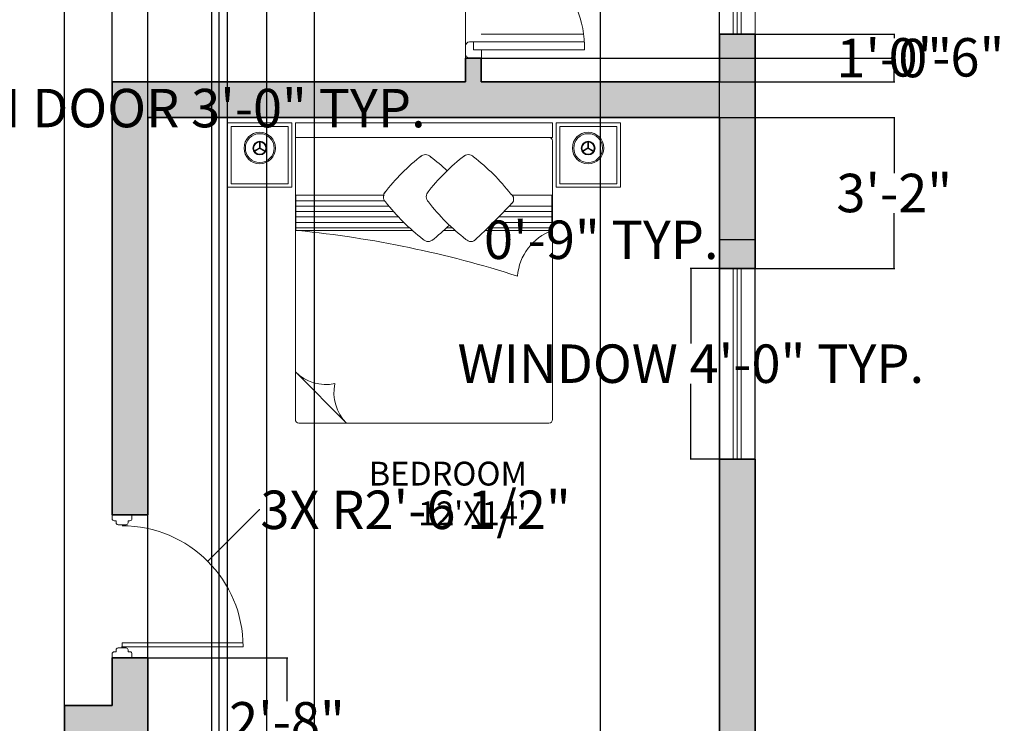
# Model space of a CAD drawing. Units: inches. Extents: x 2103 to 2702, y 2405 to 3142.
# Tile 4 of 7: x 2421 to 2669, y 2790 to 2968. Entities that reach past the tile are written whole.
import ezdxf

# ---------------------------------------------------------------- set-up
doc = ezdxf.new("R2010")
doc.units = ezdxf.units.IN
doc.linetypes.add('0', pattern=[0])
for name, color, linetype, lineweight in [('00 FURNITURE', 15, 'Continuous', 15), ('A-ANNO-DIMS', 2, 'Continuous', 18), ('A-AREA-IDEN', 7, 'Continuous', 18), ('A-WALL-PATT', 8, 'Continuous', 9), ('A_FUR 1', 5, 'Continuous', 5), ('doors', 4, 'Continuous', 18), ('WALL', 7, 'Continuous', 35), ('WINDOW', 160, '0', 5), ('windows', 4, 'Continuous', 18)]:
    doc.layers.add(name, color=color, linetype=linetype, lineweight=lineweight)
doc.layers.add('furniture', color=34, linetype='Continuous')
doc.styles.get("Standard").update_dxf_attribs({"font": 'arial.ttf'})
doc.dimstyles.get("Standard").update_dxf_attribs({"dimtxt": 9.68, "dimasz": 0.18, "dimexe": 0.18, "dimexo": 0.0625, "dimgap": 0.09, "dimtad": 0, "dimtih": 1, "dimtoh": 1, "dimdec": 1, "dimzin": 0, "dimdsep": 46, "dimlunit": 3, "dimtxsty": 'Standard', "dimcen": 0.09, "dimadec": 0, "dimazin": 0, "dimtfac": 1, "dimtdec": 1, "dimtofl": 0, "dimtmove": 0, "dimatfit": 3, "dimfxl": 1, "dimtolj": 1, "dimtzin": 0, "dimarcsym": 0})

# ---------------------------------------------------------------- blocks, each defined once
blk = doc.blocks.new('ESTSET')
at = {"layer": 'A_FUR 1'}
for p, q in [((-10.44, 4.1), (-10.44, 32.1)), ((-8.44, 4.1), (-8.44, 32.1)), ((-36.44, 6.1), (-36.44, 3.1)), ((-34.44, 6.1), (-36.44, 6.1)), ((-34.44, 4.1), (-34.44, 6.1)), ((-34.44, 4.1), (-34.44, 6.1)), ((-8.44, 4.1), (-8.44, 6.1)), ((-8.44, 6.1), (-6.44, 6.1)), ((-8.44, 4.1), (-8.44, 6.1)), ((-6.44, 6.1), (-6.44, 3.1)), ((-32.44, 4.1), (-34.44, 4.1)), ((-32.44, 4.1), (-34.44, 4.1)), ((-32.44, 3.1), (-32.44, 4.1)), ((-10.44, 3.1), (-10.44, 4.1)), ((-10.44, 4.1), (-8.44, 4.1)), ((-10.44, 4.1), (-8.44, 4.1)), ((-6.44, 2.1), (-36.44, 2.1)), ((-35.44, 2.1), (-33.44, 2.1)), ((-7.44, 2.1), (-9.44, 2.1))]:
    blk.add_line(p, q, dxfattribs=at)
for points in [[(-21.44, 2.1), (-18.67, 2.1), (-18.67, 5.1), (-20.06, 5.1)], [(-20.06, 5.1), (-20.06, -0.91)], [(-21.44, 2.1), (-21.44, -0.91), (-20.06, -0.91)]]:
    blk.add_lwpolyline(points, dxfattribs=at)
for centre, radius, start, end in [((-8.91, 6.46), 25.64, 88.9606, 185.2816), ((-35.44, 3.1), 1, 180, 270), ((-33.44, 3.1), 1, 270, 0), ((-9.44, 3.1), 1, 180, 270), ((-7.44, 3.1), 1, 270, 0)]:
    blk.add_arc(centre, radius, start, end, dxfattribs=at)
blk = doc.blocks.new('DDD')
at = {"layer": '00 FURNITURE'}
for p, q in [((-12579.77, -15859.53), (-12579.77, -15829.05)), ((-12578.77, -15859.53), (-12578.77, -15829.03)), ((-12612.02, -15857.03), (-12612.02, -15862.03)), ((-12611.02, -15857.03), (-12612.02, -15857.03)), ((-12610.52, -15858.03), (-12610.52, -15857.53)), ((-12577.52, -15858.03), (-12577.52, -15857.53)), ((-12577.02, -15857.03), (-12576.02, -15857.03)), ((-12576.02, -15857.03), (-12576.02, -15862.03)), ((-12578.77, -15859.53), (-12579.77, -15859.53)), ((-12612.02, -15862.03), (-12611.02, -15862.03)), ((-12610.52, -15861.53), (-12610.52, -15861.03)), ((-12577.52, -15861.53), (-12577.52, -15861.03)), ((-12576.02, -15862.03), (-12577.02, -15862.03))]:
    blk.add_line(p, q, dxfattribs=at)
for points in [[(-12610.52, -15861.03), (-12610.02, -15861.03, 0.414214), (-12609.52, -15860.53), (-12609.52, -15858.53, 0.414214), (-12610.02, -15858.03), (-12610.52, -15858.03)], [(-12577.52, -15861.03), (-12578.02, -15861.03, -0.414214), (-12578.52, -15860.53), (-12578.52, -15858.53, -0.414214), (-12578.02, -15858.03), (-12577.52, -15858.03)]]:
    blk.add_lwpolyline(points, format="xyb", dxfattribs=at)
for centre, radius, start, end in [((-12578.77, -15859.53), 30.5, 90, 180), ((-12611.02, -15857.53), 0.5, 0, 90), ((-12577.02, -15857.53), 0.5, 90, 180), ((-12611.02, -15861.53), 0.5, 270, 0), ((-12577.02, -15861.53), 0.5, 180, 270)]:
    blk.add_arc(centre, radius, start, end, dxfattribs=at)
blk = doc.blocks.new('window')
at = {"layer": 'furniture'}
for p, q in [((1745.13, 2764.08), (1745.13, 2716.08)), ((1754.13, 2716.08), (1754.13, 2764.08))]:
    blk.add_line(p, q, dxfattribs=at)
at = {"layer": 'WINDOW'}
for p, q in [((1748.63, 2764.08), (1748.63, 2716.08)), ((1749.63, 2764.08), (1749.63, 2716.08)), ((1750.63, 2764.08), (1750.63, 2716.08))]:
    blk.add_line(p, q, dxfattribs=at)
blk = doc.blocks.new('ventilator')
at = {"layer": 'windows'}
for p, q in [((1922.12, 2523.05), (1898.12, 2523.05)), ((1922.12, 2522.05), (1898.12, 2522.05)), ((1922.12, 2521.05), (1898.12, 2521.05))]:
    blk.add_line(p, q, dxfattribs=at)
blk.add_lwpolyline([(1898.12, 2526.55), (1898.12, 2517.55), (1922.12, 2517.55), (1922.12, 2526.55)], close=True, dxfattribs=at)
blk = doc.blocks.new('RGWTG')
at = {"layer": '00 FURNITURE'}
for p, q in [((578.23, 3473.51), (577.36, 3475.01)), ((578.23, 3473.58), (577.36, 3472.08)), ((578.36, 3473.58), (577.49, 3475.09)), ((578.36, 3473.51), (577.49, 3472)), ((578.29, 3473.62), (580.03, 3473.62)), ((578.29, 3473.47), (580.03, 3473.47)), ((521.93, 3464.58), (509.03, 3451.68)), ((509.03, 3422.63), (509.03, 3463.68)), ((509.93, 3464.58), (566.4, 3464.58)), ((557.53, 3463.84), (557.53, 3464.49)), ((557.53, 3464.49), (566.4, 3464.49)), ((558.2, 3464.49), (558.2, 3435.82)), ((559.57, 3464.49), (559.57, 3437.25)), ((560.94, 3464.49), (560.94, 3438.58)), ((562.3, 3464.49), (562.3, 3439.83)), ((563.67, 3464.49), (563.67, 3440.99)), ((565.04, 3464.49), (565.04, 3442.08)), ((566.4, 3464.58), (580.98, 3464.58)), ((566.4, 3464.49), (566.4, 3442.08)), ((566.4, 3464.49), (566.4, 3463.84)), ((580.98, 3464.58), (580.98, 3416.72)), ((558.2, 3426.48), (558.2, 3425.04)), ((509.03, 3400.68), (509.03, 3422.63)), ((558.2, 3416.13), (558.2, 3399.95)), ((580.98, 3416.72), (580.98, 3400.68)), ((559.57, 3414.75), (559.57, 3399.95)), ((560.94, 3413.39), (560.94, 3399.95)), ((562.3, 3412.04), (562.3, 3399.95)), ((563.67, 3410.72), (563.67, 3399.95)), ((580.08, 3399.78), (509.93, 3399.78)), ((557.53, 3399.95), (557.53, 3400.6)), ((566.4, 3399.95), (557.53, 3399.95)), ((566.4, 3400.6), (566.4, 3399.95)), ((578.23, 3390.78), (577.36, 3392.29)), ((578.36, 3390.86), (577.49, 3392.36)), ((578.23, 3390.86), (577.36, 3389.36)), ((578.36, 3390.78), (577.49, 3389.28)), ((578.29, 3390.9), (580.03, 3390.9)), ((578.29, 3390.74), (580.03, 3390.74))]:
    blk.add_line(p, q, dxfattribs=at)
for points in [[(568.43, 3465.48), (584.63, 3465.48), (584.63, 3481.68), (568.43, 3481.68)], [(569.33, 3466.38), (583.73, 3466.38), (583.73, 3480.78), (569.33, 3480.78)], [(580.98, 3399.78), (584.63, 3399.78), (584.63, 3464.58), (580.98, 3464.58)], [(568.43, 3398.88), (584.63, 3398.88), (584.63, 3382.68), (568.43, 3382.68)], [(569.33, 3397.98), (583.73, 3397.98), (583.73, 3383.58), (569.33, 3383.58)]]:
    blk.add_lwpolyline(points, close=True, dxfattribs=at)
for points in [[(566.52, 3464.49), (557.53, 3464.49), (557.53, 3435.08)], [(557.53, 3427.21), (557.53, 3424.3)], [(557.53, 3416.82), (557.53, 3399.95), (566.4, 3399.95), (566.4, 3409.94)]]:
    blk.add_lwpolyline(points, dxfattribs=at)
for centre, radius in [((578.29, 3473.54), 3.97), ((578.29, 3473.54), 3.63), ((578.29, 3473.54), 1.74), ((578.29, 3473.54), 1.56), ((578.29, 3390.82), 3.97), ((578.29, 3390.82), 3.63), ((578.29, 3390.82), 1.74), ((578.29, 3390.82), 1.56)]:
    blk.add_circle(centre, radius, dxfattribs=at)
for centre, radius, start, end in [((509.93, 3463.68), 0.9, 90, 180), ((529.65, 3456.88), 10.9, 135.0361, 191.9278), ((290.56, 3490.52), 268.3, 342.2214, 354.2925), ((516.73, 3443.97), 10.9, 78.0722, 134.9639), ((598.15, 3399.01), 54.32, 127.931, 142.069), ((566.05, 3440.57), 1.82, 45, 135), ((533.58, 3399.31), 54.32, 37.931, 52.069), ((556.59, 3431.11), 1.82, 135, 225), ((598.15, 3388.23), 54.32, 127.931, 142.069), ((566.05, 3429.78), 1.82, 45, 135), ((533.58, 3388.53), 54.32, 37.931, 52.069), ((574.84, 3431.77), 1.82, 315, 45), ((597.87, 3463.6), 54.32, 217.931, 224.141), ((533.28, 3463.88), 54.32, 316.32, 322.069), ((556.59, 3420.33), 1.82, 135, 225), ((574.84, 3420.99), 1.82, 315, 45), ((765.33, 3619.75), 290.45, 223.6069, 226.2326), ((533.28, 3453.1), 54.32, 307.931, 322.069), ((545.02, 3395.29), 13.35, 20.4224, 85.5825), ((565.44, 3411.05), 1.47, 225.9674, 326.8337), ((509.93, 3400.68), 0.9, 180, 270), ((580.08, 3400.68), 0.9, 270, 0)]:
    blk.add_arc(centre, radius, start, end, dxfattribs=at)
blk = doc.blocks.new('*D18')
at = {"layer": 'A-ANNO-DIMS', "color": 0, "lineweight": -2, "transparency": 16777216}
for p, q in [((2597.37, 2904.89), (2590.05, 2904.89)), ((2590.23, 2904.71), (2590.23, 2885.99)), ((2590.23, 2857.07), (2590.23, 2875.79)), ((2597.37, 2856.89), (2590.05, 2856.89))]:
    blk.add_line(p, q, dxfattribs=at)
at = {"layer": 'A-ANNO-DIMS', "color": 0, "transparency": 16777216}
for points in [[(2590.2, 2904.71), (2590.26, 2904.71), (2590.23, 2904.89)], [(2590.2, 2857.07), (2590.26, 2857.07), (2590.23, 2856.89)]]:
    blk.add_solid(points, dxfattribs=at)
at = {"layer": 'Defpoints', "color": 0, "transparency": 16777216}
for p in [(2597.43, 2904.89), (2590.23, 2856.89), (2597.43, 2856.89)]:
    blk.add_point(p, dxfattribs=at)
at = {"layer": 'A-ANNO-DIMS', "color": 0, "transparency": 16777216, "insert": (2590.23, 2880.89), "char_height": 9.68, "attachment_point": 5}
blk.add_mtext('\\A1;WINDOW 4\'-0" TYP.', dxfattribs=at)
blk = doc.blocks.new('*D19')
at = {"layer": 'A-ANNO-DIMS', "color": 0, "lineweight": -2, "transparency": 16777216}
for p, q in [((2597.43, 2904.95), (2597.43, 2912.27)), ((2606.43, 2904.95), (2606.43, 2912.27)), ((2597.43, 2912.09), (2597.25, 2912.09)), ((2606.25, 2912.09), (2597.61, 2912.09))]:
    blk.add_line(p, q, dxfattribs=at)
at = {"layer": 'A-ANNO-DIMS', "color": 0, "transparency": 16777216}
for points in [[(2597.61, 2912.12), (2597.61, 2912.06), (2597.43, 2912.09)], [(2606.25, 2912.12), (2606.25, 2912.06), (2606.43, 2912.09)]]:
    blk.add_solid(points, dxfattribs=at)
at = {"layer": 'Defpoints', "color": 0, "transparency": 16777216}
for p in [(2597.43, 2912.09), (2597.43, 2904.89), (2606.43, 2904.89)]:
    blk.add_point(p, dxfattribs=at)
at = {"layer": 'A-ANNO-DIMS', "color": 0, "transparency": 16777216, "insert": (2567.66, 2912.09), "char_height": 9.68, "attachment_point": 5}
blk.add_mtext('\\A1;0\'-9" TYP.', dxfattribs=at)
blk = doc.blocks.new('*D22')
at = {"layer": 'A-ANNO-DIMS', "color": 0, "lineweight": -2, "transparency": 16777216}
for p, q in [((2342.43, 2939.91), (2342.43, 2945.43)), ((2342.61, 2945.25), (2378.25, 2945.25)), ((2378.43, 2939.91), (2378.43, 2945.43)), ((2378.43, 2945.25), (2378.61, 2945.25))]:
    blk.add_line(p, q, dxfattribs=at)
at = {"layer": 'A-ANNO-DIMS', "color": 0, "transparency": 16777216}
for points in [[(2342.61, 2945.28), (2342.61, 2945.22), (2342.43, 2945.25)], [(2378.25, 2945.28), (2378.25, 2945.22), (2378.43, 2945.25)]]:
    blk.add_solid(points, dxfattribs=at)
at = {"layer": 'Defpoints', "color": 0, "transparency": 16777216}
for p in [(2378.43, 2945.25), (2342.43, 2939.85), (2378.43, 2939.85)]:
    blk.add_point(p, dxfattribs=at)
at = {"layer": 'A-ANNO-DIMS', "color": 0, "transparency": 16777216, "insert": (2453.03, 2945.25), "char_height": 9.68, "attachment_point": 5}
blk.add_mtext('\\A1;ROOM DOOR 3\'-0" TYP.', dxfattribs=at)
blk = doc.blocks.new('*D40')
at = {"layer": 'A-ANNO-DIMS', "color": 0, "lineweight": -2, "transparency": 16777216}
for p, q in [((2396.43, 2906.91), (2396.43, 3118.9)), ((2396.61, 3118.72), (2407.28, 3118.72)), ((2444.25, 3118.72), (2433.58, 3118.72)), ((2444.43, 2842.91), (2444.43, 3118.9))]:
    blk.add_line(p, q, dxfattribs=at)
at = {"layer": 'A-ANNO-DIMS', "color": 0, "transparency": 16777216}
for points in [[(2396.61, 3118.75), (2396.61, 3118.69), (2396.43, 3118.72)], [(2444.25, 3118.75), (2444.25, 3118.69), (2444.43, 3118.72)]]:
    blk.add_solid(points, dxfattribs=at)
at = {"layer": 'Defpoints', "color": 0, "transparency": 16777216}
for p in [(2444.43, 3118.72), (2396.43, 2906.85), (2444.43, 2842.85)]:
    blk.add_point(p, dxfattribs=at)
at = {"layer": 'A-ANNO-DIMS', "color": 0, "transparency": 16777216, "insert": (2420.43, 3118.72), "char_height": 9.68, "attachment_point": 5}
blk.add_mtext('\\A1;4\'-0"', dxfattribs=at)
blk = doc.blocks.new('*D44')
at = {"layer": 'A-ANNO-DIMS', "color": 0, "lineweight": -2, "transparency": 16777216}
for p, q in [((2471.43, 2560.91), (2471.43, 3118.9)), ((2471.61, 3118.72), (2483.25, 3118.72)), ((2483.43, 2560.91), (2483.43, 3118.9)), ((2483.43, 3118.72), (2483.61, 3118.72))]:
    blk.add_line(p, q, dxfattribs=at)
at = {"layer": 'A-ANNO-DIMS', "color": 0, "transparency": 16777216}
for points in [[(2471.61, 3118.75), (2471.61, 3118.69), (2471.43, 3118.72)], [(2483.25, 3118.75), (2483.25, 3118.69), (2483.43, 3118.72)]]:
    blk.add_solid(points, dxfattribs=at)
at = {"layer": 'Defpoints', "color": 0, "transparency": 16777216}
for p in [(2483.43, 3118.72), (2471.43, 2560.85), (2483.43, 2560.85)]:
    blk.add_point(p, dxfattribs=at)
at = {"layer": 'A-ANNO-DIMS', "color": 0, "transparency": 16777216, "insert": (2496.11, 3118.72), "char_height": 9.68, "attachment_point": 5}
blk.add_mtext('\\A1;1\'-0"', dxfattribs=at)
blk = doc.blocks.new('*D45')
at = {"layer": 'A-ANNO-DIMS', "color": 0, "lineweight": -2, "transparency": 16777216}
for p, q in [((2567.43, 2560.91), (2567.43, 3118.9)), ((2567.61, 3118.72), (2569.39, 3118.72)), ((2597.25, 3118.72), (2595.47, 3118.72)), ((2597.43, 2560.91), (2597.43, 3118.9))]:
    blk.add_line(p, q, dxfattribs=at)
at = {"layer": 'A-ANNO-DIMS', "color": 0, "transparency": 16777216}
for points in [[(2567.61, 3118.75), (2567.61, 3118.69), (2567.43, 3118.72)], [(2597.25, 3118.75), (2597.25, 3118.69), (2597.43, 3118.72)]]:
    blk.add_solid(points, dxfattribs=at)
at = {"layer": 'Defpoints', "color": 0, "transparency": 16777216}
for p in [(2597.43, 3118.72), (2567.43, 2560.85), (2597.43, 2560.85)]:
    blk.add_point(p, dxfattribs=at)
at = {"layer": 'A-ANNO-DIMS', "color": 0, "transparency": 16777216, "insert": (2582.43, 3118.72), "char_height": 9.68, "attachment_point": 5}
blk.add_mtext('\\A1;2\'-6"', dxfattribs=at)
blk = doc.blocks.new('*D50')
at = {"layer": 'A-ANNO-DIMS', "color": 0, "lineweight": -2, "transparency": 16777216}
for p, q in [((2453.43, 2569.91), (2453.43, 3118.9)), ((2453.61, 3118.72), (2461.48, 3118.72)), ((2495.25, 3118.72), (2487.38, 3118.72)), ((2495.43, 2569.91), (2495.43, 3118.9))]:
    blk.add_line(p, q, dxfattribs=at)
at = {"layer": 'A-ANNO-DIMS', "color": 0, "transparency": 16777216}
for points in [[(2453.61, 3118.75), (2453.61, 3118.69), (2453.43, 3118.72)], [(2495.25, 3118.75), (2495.25, 3118.69), (2495.43, 3118.72)]]:
    blk.add_solid(points, dxfattribs=at)
at = {"layer": 'Defpoints', "color": 0, "transparency": 16777216}
for p in [(2495.43, 3118.72), (2453.43, 2569.85), (2495.43, 2569.85)]:
    blk.add_point(p, dxfattribs=at)
at = {"layer": 'A-ANNO-DIMS', "color": 0, "transparency": 16777216, "insert": (2474.43, 3118.72), "char_height": 9.68, "attachment_point": 5}
blk.add_mtext('\\A1;3\'-6"', dxfattribs=at)
blk = doc.blocks.new('*D59')
at = {"layer": 'A-ANNO-DIMS', "color": 0, "lineweight": -2, "transparency": 16777216}
for p, q in [((2597.49, 2963.85), (2641.66, 2963.85)), ((2641.48, 2963.67), (2641.48, 2962.88)), ((2641.48, 2952.03), (2641.48, 2952.81)), ((2597.49, 2951.85), (2641.66, 2951.85))]:
    blk.add_line(p, q, dxfattribs=at)
at = {"layer": 'A-ANNO-DIMS', "color": 0, "transparency": 16777216}
for points in [[(2641.45, 2963.67), (2641.51, 2963.67), (2641.48, 2963.85)], [(2641.45, 2952.03), (2641.51, 2952.03), (2641.48, 2951.85)]]:
    blk.add_solid(points, dxfattribs=at)
at = {"layer": 'Defpoints', "color": 0, "transparency": 16777216}
for p in [(2597.43, 2963.85), (2641.48, 2963.85), (2597.43, 2951.85)]:
    blk.add_point(p, dxfattribs=at)
at = {"layer": 'A-ANNO-DIMS', "color": 0, "transparency": 16777216, "insert": (2641.48, 2957.85), "char_height": 9.68, "attachment_point": 5}
blk.add_mtext('\\A1;1\'-0"', dxfattribs=at)
blk = doc.blocks.new('*D60')
at = {"layer": 'A-ANNO-DIMS', "color": 0, "lineweight": -2, "transparency": 16777216}
for p, q in [((2597.49, 2942.85), (2641.66, 2942.85)), ((2641.48, 2942.67), (2641.48, 2928.9)), ((2641.48, 2905.07), (2641.48, 2918.83)), ((2597.49, 2904.89), (2641.66, 2904.89))]:
    blk.add_line(p, q, dxfattribs=at)
at = {"layer": 'A-ANNO-DIMS', "color": 0, "transparency": 16777216}
for points in [[(2641.45, 2942.67), (2641.51, 2942.67), (2641.48, 2942.85)], [(2641.45, 2905.07), (2641.51, 2905.07), (2641.48, 2904.89)]]:
    blk.add_solid(points, dxfattribs=at)
at = {"layer": 'Defpoints', "color": 0, "transparency": 16777216}
for p in [(2597.43, 2942.85), (2641.48, 2942.85), (2597.43, 2904.89)]:
    blk.add_point(p, dxfattribs=at)
at = {"layer": 'A-ANNO-DIMS', "color": 0, "transparency": 16777216, "insert": (2641.48, 2923.87), "char_height": 9.68, "attachment_point": 5}
blk.add_mtext('\\A1;3\'-2"', dxfattribs=at)
blk = doc.blocks.new('*D66')
at = {"layer": 'A-ANNO-DIMS', "color": 0, "lineweight": -2, "transparency": 16777216}
for p, q in [((2384.43, 2794.91), (2384.43, 3118.9)), ((2384.61, 3118.72), (2395.28, 3118.72)), ((2432.25, 3118.72), (2421.58, 3118.72)), ((2432.43, 2794.91), (2432.43, 3118.9))]:
    blk.add_line(p, q, dxfattribs=at)
at = {"layer": 'A-ANNO-DIMS', "color": 0, "transparency": 16777216}
for points in [[(2384.61, 3118.75), (2384.61, 3118.69), (2384.43, 3118.72)], [(2432.25, 3118.75), (2432.25, 3118.69), (2432.43, 3118.72)]]:
    blk.add_solid(points, dxfattribs=at)
at = {"layer": 'Defpoints', "color": 0, "transparency": 16777216}
for p in [(2384.43, 3118.72), (2384.43, 2794.85), (2432.43, 2794.85)]:
    blk.add_point(p, dxfattribs=at)
at = {"layer": 'A-ANNO-DIMS', "color": 0, "transparency": 16777216, "insert": (2408.43, 3118.72), "char_height": 9.68, "attachment_point": 5}
blk.add_mtext('\\A1;4\'-0"', dxfattribs=at)
blk = doc.blocks.new('*D67')
at = {"layer": 'A-ANNO-DIMS', "color": 0, "lineweight": -2, "transparency": 16777216}
for p, q in [((2469.43, 2999.78), (2469.43, 2411.62)), ((2473.43, 2999.78), (2473.43, 2411.62)), ((2469.43, 2411.8), (2469.25, 2411.8)), ((2473.25, 2411.8), (2469.61, 2411.8))]:
    blk.add_line(p, q, dxfattribs=at)
at = {"layer": 'A-ANNO-DIMS', "color": 0, "transparency": 16777216}
for points in [[(2469.61, 2411.83), (2469.61, 2411.77), (2469.43, 2411.8)], [(2473.25, 2411.83), (2473.25, 2411.77), (2473.43, 2411.8)]]:
    blk.add_solid(points, dxfattribs=at)
at = {"layer": 'Defpoints', "color": 0, "transparency": 16777216}
for p in [(2469.43, 2999.85), (2473.43, 2999.85), (2469.43, 2411.8)]:
    blk.add_point(p, dxfattribs=at)
at = {"layer": 'A-ANNO-DIMS', "color": 0, "transparency": 16777216, "insert": (2456.29, 2411.8), "char_height": 9.68, "attachment_point": 5}
blk.add_mtext('\\A1;0\'-4"', dxfattribs=at)
blk = doc.blocks.new('*D70')
at = {"layer": 'A-ANNO-DIMS', "color": 0, "lineweight": -2, "transparency": 16777216}
for p, q in [((2537.49, 2957.85), (2641.66, 2957.85)), ((2641.48, 2957.85), (2641.48, 2958.03)), ((2641.48, 2958.03), (2641.66, 2958.03)), ((2641.48, 2952.03), (2641.48, 2957.67)), ((2537.49, 2951.85), (2641.66, 2951.85))]:
    blk.add_line(p, q, dxfattribs=at)
at = {"layer": 'A-ANNO-DIMS', "color": 0, "transparency": 16777216}
for points in [[(2641.45, 2957.67), (2641.51, 2957.67), (2641.48, 2957.85)], [(2641.45, 2952.03), (2641.51, 2952.03), (2641.48, 2951.85)]]:
    blk.add_solid(points, dxfattribs=at)
at = {"layer": 'Defpoints', "color": 0, "transparency": 16777216}
for p in [(2537.43, 2957.85), (2641.48, 2957.85), (2537.43, 2951.85)]:
    blk.add_point(p, dxfattribs=at)
at = {"layer": 'A-ANNO-DIMS', "color": 0, "transparency": 16777216, "insert": (2654.62, 2958.03), "char_height": 9.68, "attachment_point": 5}
blk.add_mtext('\\A1;0\'-6"', dxfattribs=at)
blk = doc.blocks.new('*D71')
at = {"layer": 'A-ANNO-DIMS', "color": 0, "lineweight": -2, "transparency": 16777216}
for p, q in [((2453.49, 2806.85), (2488.66, 2806.85)), ((2488.48, 2806.67), (2488.48, 2795.88)), ((2488.48, 2775.03), (2488.48, 2785.81)), ((2453.49, 2774.85), (2488.66, 2774.85))]:
    blk.add_line(p, q, dxfattribs=at)
at = {"layer": 'A-ANNO-DIMS', "color": 0, "transparency": 16777216}
for points in [[(2488.45, 2806.67), (2488.51, 2806.67), (2488.48, 2806.85)], [(2488.45, 2775.03), (2488.51, 2775.03), (2488.48, 2774.85)]]:
    blk.add_solid(points, dxfattribs=at)
at = {"layer": 'Defpoints', "color": 0, "transparency": 16777216}
for p in [(2453.43, 2806.85), (2453.43, 2774.85), (2488.48, 2774.85)]:
    blk.add_point(p, dxfattribs=at)
at = {"layer": 'A-ANNO-DIMS', "color": 0, "transparency": 16777216, "insert": (2488.48, 2790.85), "char_height": 9.68, "attachment_point": 5}
blk.add_mtext('\\A1;2\'-8"', dxfattribs=at)
blk = doc.blocks.new('*D79')
at = {"layer": 'A-ANNO-DIMS', "color": 0, "lineweight": -2, "transparency": 16777216}
for p, q in [((2481.44, 2844.1), (2468.62, 2831.29)), ((2481.62, 2844.1), (2481.44, 2844.1)), ((2446.84, 2809.6), (2447.02, 2809.6)), ((2446.93, 2809.51), (2446.93, 2809.69))]:
    blk.add_line(p, q, dxfattribs=at)
at = {"layer": 'A-ANNO-DIMS', "color": 0, "transparency": 16777216}
blk.add_solid([(2468.6, 2831.31), (2468.65, 2831.27), (2468.5, 2831.16)], dxfattribs=at)
at = {"layer": 'Defpoints', "color": 0, "transparency": 16777216}
for p in [(2468.5, 2831.16), (2446.93, 2809.6)]:
    blk.add_point(p, dxfattribs=at)
at = {"layer": 'A-ANNO-DIMS', "color": 0, "transparency": 16777216, "insert": (2520.88, 2844.1), "char_height": 9.68, "attachment_point": 5}
blk.add_mtext('\\A1;3X R2\'-6 1/2"', dxfattribs=at)

msp = doc.modelspace()

# ---------------------------------------------------------------- hatches: boundary and pattern name
at = {"layer": 'A-WALL-PATT'}
h = msp.add_hatch(color=256, dxfattribs=at)
h.dxf.hatch_style = 1
h.paths.add_polyline_path([(2342.43, 2911.85), (2342.43, 2915.85), (2255.43, 2915.85), (2255.43, 2976.23), (2246.43, 2976.23), (2246.43, 2840.19), (2255.43, 2840.19), (2255.43, 2854.85), (2315.43, 2854.85), (2315.43, 2845.85), (2319.43, 2845.85), (2319.43, 2858.85), (2255.43, 2858.85), (2255.43, 2906.85), (2342.43, 2906.85)])
h.paths.add_polyline_path([(2384.43, 2794.85), (2319.43, 2794.85), (2319.43, 2815.85), (2315.43, 2815.85), (2315.43, 2794.85), (2255.43, 2794.85), (2255.43, 2816.19), (2246.43, 2816.19), (2246.43, 2753.7), (2255.43, 2753.7), (2255.43, 2785.85), (2384.43, 2785.85)])
h.paths.add_polyline_path([(2606.43, 2963.85), (2597.43, 2963.85), (2597.43, 2951.85), (2537.43, 2951.85), (2537.43, 2957.85), (2533.43, 2957.85), (2533.43, 2951.85), (2469.43, 2951.85), (2444.43, 2951.85), (2444.43, 2842.85), (2449.43, 2842.85), (2453.43, 2842.85), (2453.43, 2942.85), (2597.43, 2942.85), (2597.43, 2904.89), (2606.43, 2904.89)])
h.paths.add_polyline_path([(2606.43, 3019.85), (2597.43, 3019.85), (2597.43, 3003.85), (2537.43, 3003.85), (2537.43, 3015.85), (2533.43, 3015.85), (2533.43, 2987.85), (2537.43, 2987.85), (2537.43, 2999.85), (2597.43, 2999.85), (2597.43, 2987.85), (2606.43, 2987.85)])
h.paths.add_polyline_path([(2606.43, 2856.89), (2597.43, 2856.89), (2597.43, 2774.85), (2552.43, 2774.85), (2552.43, 2765.85), (2597.43, 2765.85), (2597.43, 2749.52), (2606.43, 2749.52)])
h.paths.add_polyline_path([(2522.43, 2774.85), (2453.43, 2774.85), (2453.43, 2806.85), (2444.43, 2806.85), (2444.43, 2794.85), (2432.43, 2794.85), (2432.43, 2785.85), (2444.43, 2785.85), (2444.43, 2765.85), (2453.43, 2765.85), (2509.43, 2765.85), (2509.43, 2705.85), (2498.43, 2705.85), (2498.43, 2701.85), (2597.43, 2701.85), (2597.43, 2678.29), (2606.43, 2678.29), (2606.43, 2725.52), (2597.43, 2725.52), (2597.43, 2705.85), (2513.43, 2705.85), (2513.43, 2765.85), (2522.43, 2765.85)])
h.paths.add_polyline_path([(2255.43, 2705.7), (2246.43, 2705.7), (2246.43, 2646.55), (2255.43, 2646.55)])
h.paths.add_polyline_path([(2255.43, 2598.55), (2246.43, 2598.55), (2246.43, 2560.85), (2309.13, 2560.85), (2309.13, 2569.85), (2309.13, 2569.85), (2255.43, 2569.85)])
h.paths.add_polyline_path([(2495.43, 2569.85), (2495.43, 2569.85), (2453.43, 2569.85), (2453.43, 2701.85), (2462.43, 2701.85), (2462.43, 2705.85), (2444.43, 2705.85), (2444.43, 2569.85), (2432.43, 2569.85), (2432.43, 2564.45), (2432.43, 2564.45), (2432.43, 2560.85), (2495.43, 2560.85)])
h.paths.add_polyline_path([(2384.43, 2569.85), (2357.13, 2569.85), (2357.13, 2560.85), (2384.43, 2560.85)])
h.paths.add_polyline_path([(2606.43, 2630.29), (2597.43, 2630.29), (2597.43, 2569.85), (2543.43, 2569.85), (2543.43, 2560.85), (2597.43, 2560.85), (2597.43, 2455.85), (2450.43, 2455.85), (2450.43, 2446.85), (2606.43, 2446.85)])

# ---------------------------------------------------------------- linework, layer by layer
at = {"layer": 'doors'}
msp.add_line((2537.43, 2963.85), (2563.24, 2963.85), dxfattribs=at)
at = {"layer": 'WALL'}
for p, q in [((2597.43, 2963.85), (2597.43, 2951.85)), ((2597.43, 2963.85), (2606.43, 2963.85)), ((2606.43, 2963.85), (2606.43, 2904.89)), ((2533.43, 2957.85), (2537.43, 2957.85)), ((2533.43, 2957.85), (2533.43, 2951.85)), ((2537.43, 2957.85), (2537.43, 2951.85)), ((2473.43, 2951.85), (2444.43, 2951.85)), ((2444.43, 2951.85), (2444.43, 2842.85)), ((2469.43, 2951.85), (2533.43, 2951.85)), ((2537.43, 2951.85), (2597.43, 2951.85)), ((2453.43, 2942.85), (2597.43, 2942.85)), ((2453.43, 2942.85), (2453.43, 2842.85)), ((2597.43, 2942.85), (2597.43, 2904.89)), ((2597.43, 2904.89), (2606.43, 2904.89)), ((2597.43, 2856.89), (2606.43, 2856.89)), ((2597.43, 2856.89), (2597.43, 2774.85)), ((2606.43, 2856.89), (2606.43, 2749.52)), ((2444.43, 2842.85), (2453.43, 2842.85)), ((2444.43, 2806.85), (2453.43, 2806.85)), ((2444.43, 2806.85), (2444.43, 2794.85)), ((2453.43, 2806.85), (2453.43, 2774.85)), ((2432.43, 2794.85), (2432.43, 2785.85)), ((2432.43, 2794.85), (2444.43, 2794.85))]:
    msp.add_line(p, q, dxfattribs=at)

# ---------------------------------------------------------------- block references
at = {"layer": '00 FURNITURE', "rotation": 89.99999999999999}
msp.add_blockref('RGWTG', (5955.17, 2356.89), dxfattribs=at)
at = {"layer": 'doors'}
for name, p, rotation in [('ESTSET', (2531.37, 2951.47), 270), ('DDD', (18306.46, -9769.18), 269.9999999934867)]:
    msp.add_blockref(name, p, dxfattribs=dict(at, rotation=rotation))
at = {"layer": 'windows'}
for name, p, rotation in [('ventilator', (79.88, 4885.97), 270), ('window', (4351.56, 5620.97), 180)]:
    msp.add_blockref(name, p, dxfattribs=dict(at, rotation=rotation))

# ---------------------------------------------------------------- texts
at = {"layer": 'A-AREA-IDEN', "insert": (2548.93, 2856.21), "char_height": 7.1875, "attachment_point": 3}
msp.add_mtext_dynamic_manual_height_columns(" {\\H0.83478x;BEDROOM  12'X14'}", width=41.3807, gutter_width=12.5, heights=[0], dxfattribs=at)

# ---------------------------------------------------------------- dimensions: what is measured, and where the dimension line sits
at = {"layer": 'A-ANNO-DIMS'}
for base, p1, p2, picture, middle in [((2384.43, 3118.72), (2432.43, 2794.85), (2384.43, 2794.85), '*D66', (2408.43, 3118.72)), ((2444.43, 3118.72), (2396.43, 2906.85), (2444.43, 2842.85), '*D40', (2420.43, 3118.72)), ((2495.43, 3118.72), (2453.43, 2569.85), (2495.43, 2569.85), '*D50', (2474.43, 3118.72)), ((2483.43, 3118.72), (2471.43, 2560.85), (2483.43, 2560.85), '*D44', (2496.11, 3118.72)), ((2597.43, 3118.72), (2567.43, 2560.85), (2597.43, 2560.85), '*D45', (2582.43, 3118.72)), ((2469.43, 2411.8), (2473.43, 2999.85), (2469.43, 2999.85), '*D67', (2456.29, 2411.8))]:
    dim = msp.add_linear_dim(base=base, p1=p1, p2=p2, dimstyle='Standard', override={"dimdec": 1, "dimlfac": 1, "dimrnd": 0, "dimzin": 1, "dimdsep": 46, "dimlunit": 4, "dimfrac": 2}, dxfattribs=at)
    dim.commit()
    dim.dimension.update_dxf_attribs({"geometry": picture, "text_midpoint": middle})
for base, p1, p2, angle, text, picture, middle in [((2378.43, 2945.25), (2342.43, 2939.85), (2378.43, 2939.85), 360, 'ROOM DOOR <> TYP.', '*D22', (2453.03, 2945.25)), ((2597.43, 2912.09), (2606.43, 2904.89), (2597.43, 2904.89), 180, '<> TYP.', '*D19', (2567.66, 2912.09)), ((2590.23, 2856.89), (2597.43, 2904.89), (2597.43, 2856.89), 270, 'WINDOW <> TYP.', '*D18', (2590.23, 2880.89))]:
    dim = msp.add_linear_dim(base=base, p1=p1, p2=p2, angle=angle, text=text, dimstyle='Standard', override={"dimdec": 1, "dimlfac": 1, "dimrnd": 0, "dimzin": 1, "dimdsep": 46, "dimlunit": 4, "dimfrac": 2}, dxfattribs=at)
    dim.commit()
    dim.dimension.update_dxf_attribs({"geometry": picture, "text_midpoint": middle})
for base, p1, p2, angle, picture, middle in [((2641.48, 2957.85), (2537.43, 2951.85), (2537.43, 2957.85), 90, '*D70', (2654.62, 2958.03)), ((2641.48, 2963.85), (2597.43, 2951.85), (2597.43, 2963.85), 90, '*D59', (2641.48, 2957.85)), ((2641.48, 2942.85), (2597.43, 2904.89), (2597.43, 2942.85), 90, '*D60', (2641.48, 2923.87)), ((2488.48, 2774.85), (2453.43, 2806.85), (2453.43, 2774.85), 270, '*D71', (2488.48, 2790.85))]:
    dim = msp.add_linear_dim(base=base, p1=p1, p2=p2, angle=angle, dimstyle='Standard', override={"dimdec": 1, "dimlfac": 1, "dimrnd": 0, "dimzin": 1, "dimdsep": 46, "dimlunit": 4, "dimfrac": 2}, dxfattribs=at)
    dim.commit()
    dim.dimension.update_dxf_attribs({"geometry": picture, "text_midpoint": middle})
dim = msp.add_radius_dim(center=(2446.93, 2809.6), mpoint=(2468.5, 2831.16), text='3X <>', dimstyle='Standard', override={"dimdec": 1, "dimlfac": 1, "dimrnd": 0, "dimzin": 1, "dimdsep": 46, "dimlunit": 4, "dimfrac": 2}, dxfattribs=at)
dim.commit()
dim.dimension.update_dxf_attribs({"geometry": '*D79', "text_midpoint": (2520.88, 2844.1), "dimtype": 164})

doc.saveas('drawing.dxf')
